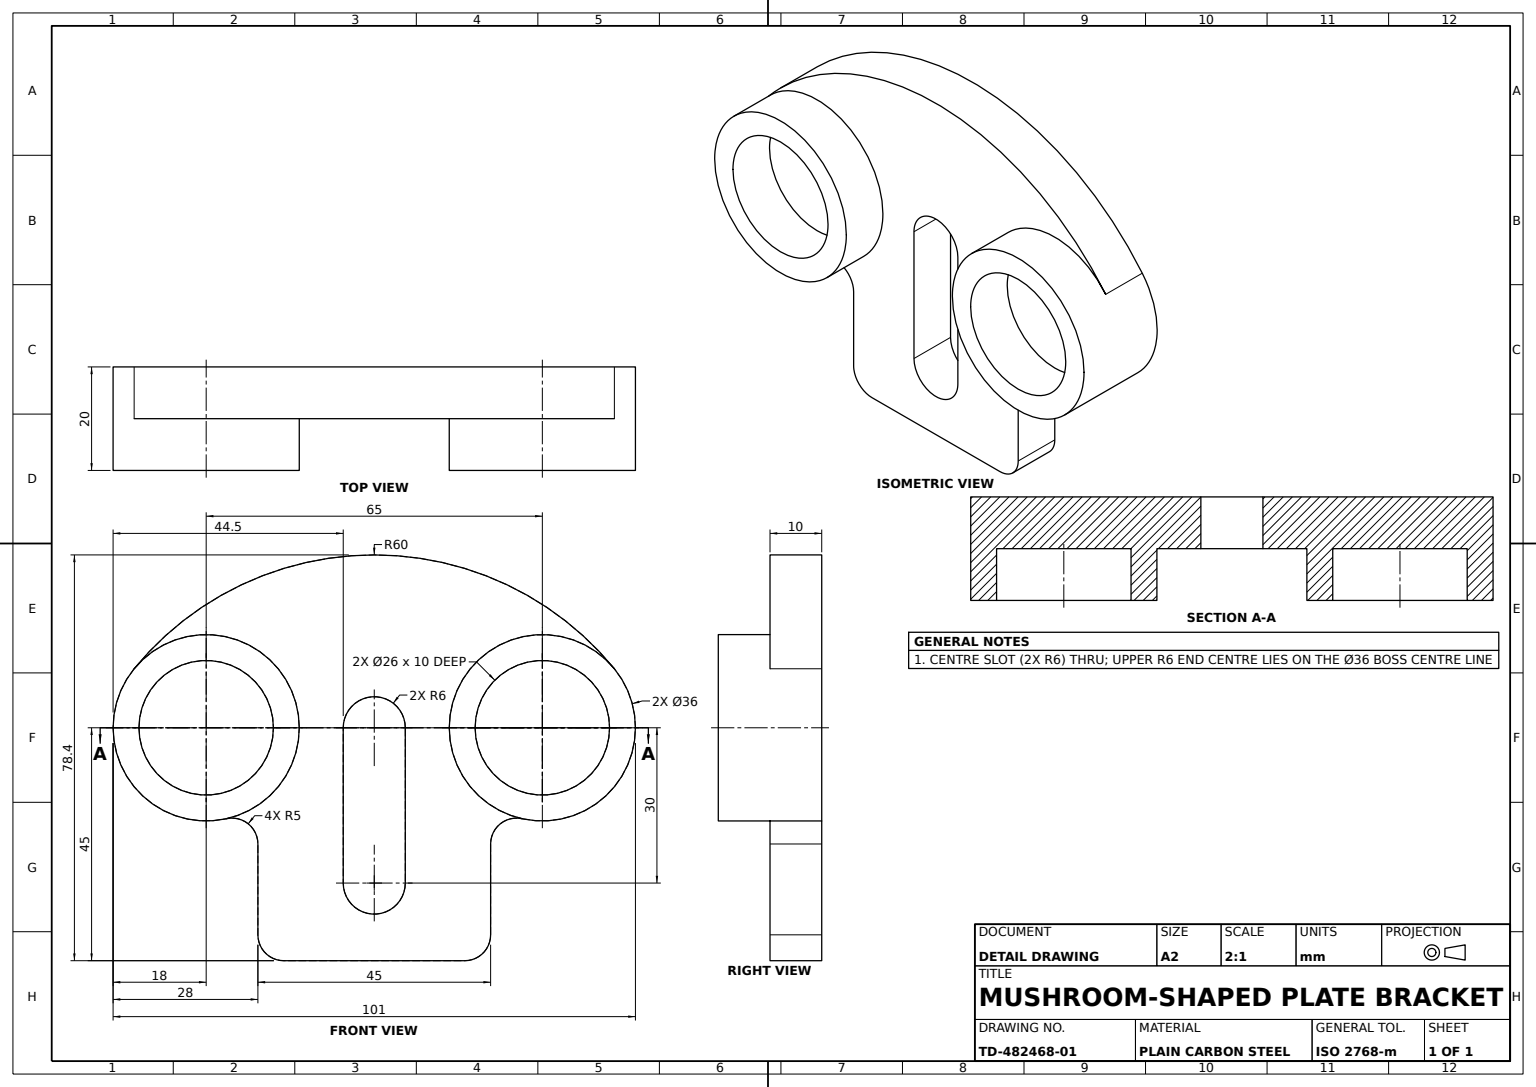
SolidWorks part; units mm, degrees
material "Plain Carbon Steel"
ref_plane "Front Plane" through (0, 0, 0) normal (0, 0, 1) x (1, 0, 0)
ref_plane "Top Plane" through (0, 0, 0) normal (0, 1, 0) x (1, 0, 0)
ref_plane "Right Plane" through (0, 0, 0) normal (1, 0, 0) x (0, 0, -1)
sketch "Lobed Base Sketch" plane through (0, 0, 0) normal (0, 0, 1) x (1, 0, 0)
  line L0 (0, 0) -> (65, 0)
  line L1 (32.5, 0) -> (32.5, -45)
  line L2 (15, -45) -> (50, -45)
  line L3 (55, -40) -> (55, -22.4499)
  line L4 (10, -40) -> (10, -22.4499)
  arc A0 (-13.9286, 11.4015) -> (3.913, -17.5695) centre (0, 0) ccw
  arc A1 (61.087, -17.5695) -> (78.9286, 11.4015) centre (65, 0) ccw
  arc A2 (-13.9286, 11.4015) -> (78.9286, 11.4015) centre (32.5, -26.6036) cw
  arc A3 (55, -22.4499) -> (61.087, -17.5695) centre (60, -22.4499) cw
  arc A4 (10, -22.4499) -> (3.913, -17.5695) centre (5, -22.4499) ccw
  arc A5 (50, -45) -> (55, -40) centre (50, -40) ccw
  arc A6 (15, -45) -> (10, -40) centre (15, -40) cw
  point P13 (32.5, -45)
  point P19 (55, -45)
  dimension "D1" = 18
  dimension "D3" = 18
  dimension "D5" = 60
  dimension "D7" = 5
  dimension "D8" = 5
  dimension "D2" = 65
  dimension "D4" = 45
  dimension "D6" = 22.5
extrude "Lobed Base Plate" add sketch "Lobed Base Sketch" along normal blind 10
sketch "Round Bosses Sketch" plane through (0, 0, 10) normal (0, 0, 1) x (1, 0, 0)
  circle A0 centre (0, 0) radius 18
  circle A1 centre (65, 0) radius 18
  dimension "D1" = 36
  dimension "D2" = 36
extrude "Round Bosses 2xØ36" add sketch "Round Bosses Sketch" along normal blind 10
sketch "Boss Bores Sketch" plane through (0, 0, 20) normal (0, 0, 1) x (1, 0, 0)
  circle A0 centre (0, 0) radius 13
  circle A1 centre (65, 0) radius 13
  dimension "D1" = 13
  dimension "D2" = 13
extrude "Boss Bores 2xØ13" cut sketch "Boss Bores Sketch" against normal blind 10
sketch "Center Slot Sketch" plane through (0, 0, 10) normal (0, 0, 1) x (1, 0, 0)
  line L0 (0, 0) -> (65, 0)
  line L1 (32.5, 0) -> (32.5, -30)
  line L2 (26.5, 0) -> (26.5, -30)
  line L3 (38.5, 0) -> (38.5, -30)
  arc A0 (38.5, 0) -> (26.5, 0) centre (32.5, 0) ccw
  arc A1 (26.5, -30) -> (38.5, -30) centre (32.5, -30) ccw
  dimension "D2" = 6
  dimension "D3" = 6
  dimension "D5" = 30
extrude "Center Slot" cut sketch "Center Slot Sketch" against normal blind 20
